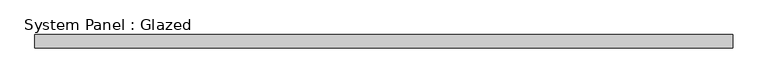
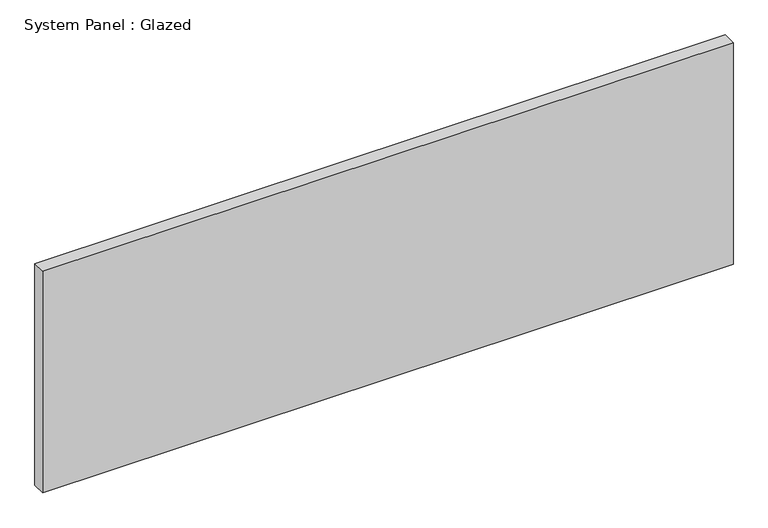
"""IFC4 building model written with IfcOpenShell, lengths in millimetres: plate geometry, System Panel : Glazed."""

from ifc_helpers import new_model, si_unit, origin, origin_with_axes, place, context, project, spatial, polyline, outline, extrude, source, transform, mapped, element, save


def system_panel_glazed_201df7ca(model_context):
    return source(origin(), model_context, "Body", "SweptSolid", [
        extrude(outline(polyline([(655.1083334, 19.05), (-655.1083334, 19.05), (-655.1083334, 44.45), (655.1083334, 44.45), (655.1083334, 19.05)])), origin_with_axes(), (0.0, 0.0, 1.0), 444.5),
    ])


if __name__ == "__main__":
    model = new_model("IFC4")
    model_context = context("Model", 3, world=origin())
    ifc_project = project(units=[si_unit("LENGTHUNIT", "METRE", prefix="MILLI")], contexts=[model_context])
    site = spatial("IfcSite", under=ifc_project)
    building = spatial("IfcBuilding", under=site)
    placement = place(None, origin())
    system_panel_glazed_shape = system_panel_glazed_201df7ca(model_context)
    element("IfcPlate", 1, ObjectType="System Panel : Glazed", at=placement, inside=building, context=model_context, shape_type="MappedRepresentation", body=[
        mapped(system_panel_glazed_shape, transform((0.0, 0.0, 0.0), x_axis=(1.0, 0.0, 0.0), y_axis=(0.0, 1.0, 0.0), z_axis=(0.0, 0.0, 1.0))),
    ])
    save(model, "model.ifc")

# Revit data of these elements
# Type "System Panel : Glazed"
#   Construction Type Id = "GSP4R"
#   Analytic Construction = "1/8 in Pilkington single glazing"
#   Visual Light Transmittance = 0.9
#   Solar Heat Gain Coefficient = 0.86
#   Heat Transfer Coefficient (U) = 1.18115 BTU/(h·ft²·°F)
#   Define Thermal Properties by = 1
# Element 1 (IfcPlate, "System Panel : Glazed")
#   Materials on its faces: "glass panel 223"
# Materials
#   "glass panel 223": class "Generic", colour RGB 120 120 120, transparency 0, Cost = 0
